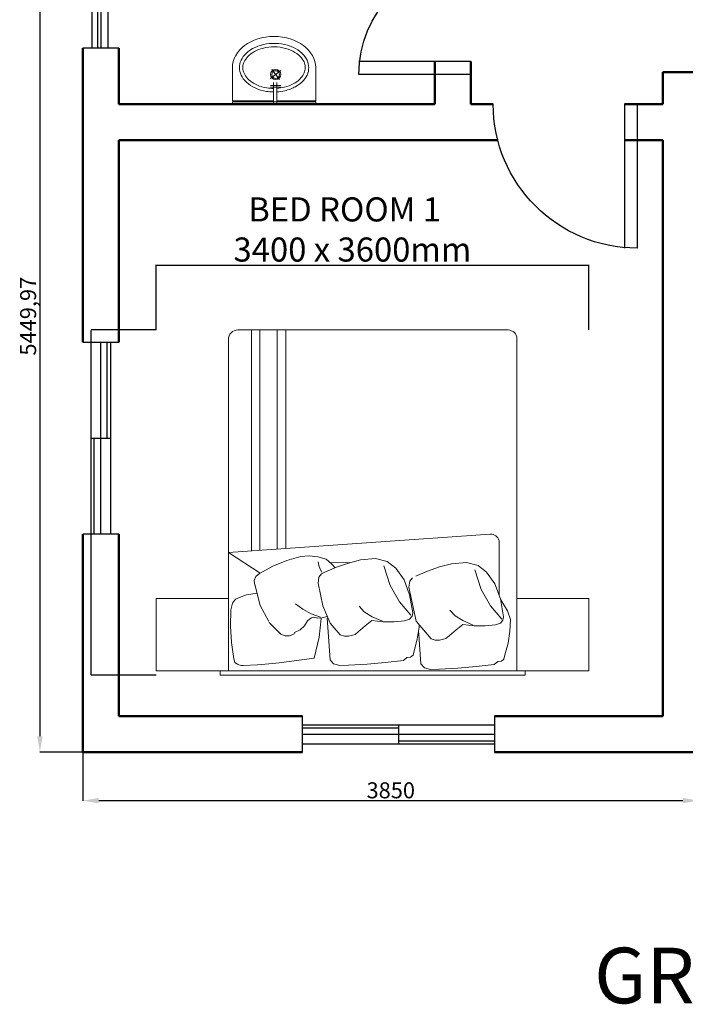
# Model space of a CAD drawing. Units: millimetres. Extents: x -857 to 54106, y -13666 to 13947.
# Tile 2 of 41: x 3174 to 7333, y 2329 to 8482. Entities that reach past the tile are written whole.
import ezdxf

# ---------------------------------------------------------------- set-up
doc = ezdxf.new("R2010")
doc.units = ezdxf.units.MM
for name, color, linetype, lineweight in [('A-ANNO-DIMS', 2, 'Continuous', 18), ('A-ANNO-TEXT', 7, 'Continuous', 25), ('A-AREA-IDEN', 3, 'Continuous', 18), ('A-DOOR', 1, 'Continuous', 25), ('A-FLOR-FIXT', 8, 'Continuous', 18), ('A-FURN', 21, 'Continuous', 18), ('A-FURNITURE', 25, 'Continuous', 9), ('A-GLAZ', 4, 'Continuous', 25), ('A-SANITARY FITTINGS', 25, 'Continuous', 15), ('A-WALL', 7, 'Continuous', 50)]:
    doc.layers.add(name, color=color, linetype=linetype, lineweight=lineweight)
doc.styles.get("Standard").update_dxf_attribs({"font": 'arial.ttf'})
doc.dimstyles.new('ISO-25', dxfattribs={"dimtxt": 2.5, "dimasz": 2.5, "dimexe": 1.25, "dimexo": 0.625, "dimtad": 1, "dimtxsty": 'Standard', "dimcen": 2.5, "dimadec": 0, "dimazin": 0, "dimtfac": 1, "dimtmove": 0, "dimatfit": 3, "dimfxl": 1, "dimarcsym": 0})

# ---------------------------------------------------------------- blocks, each defined once
blk = doc.blocks.new('A$C06e6df2d')
at = {"layer": 'A-FURNITURE'}
for p, q in [((-73.01, 70.89), (-16.87, 70.89)), ((-70.22, 24.92), (-70.22, 70.89)), ((-68.43, 25.04), (-68.43, 70.89)), ((-64.83, 25.3), (-64.83, 70.89)), ((-63.04, 25.42), (-63.04, 70.89)), ((-75.01, 24.58), (-75.01, 68.89)), ((-15.01, 0), (-15.01, 69.09)), ((-75.01, 24.58), (-20.56, 28.42)), ((-18.69, 15.78), (-18.71, 27.06)), ((-68.39, 20.29), (-75.01, 24.58)), ((-75.01, 24.58), (-75.01, 0)), ((-65.73, 21.73), (-62.87, 22.91)), ((-62.87, 22.91), (-59.95, 23.77)), ((-59.95, 23.77), (-58.19, 23.92)), ((-58.19, 23.92), (-56.43, 23.73)), ((-56.43, 23.73), (-54.68, 23.22)), ((-56.16, 21.87), (-56.3, 22.64)), ((-54.68, 23.22), (-54.09, 22.72)), ((-54.09, 22.72), (-53.51, 22.17)), ((-50.02, 22.42), (-47.49, 23.05)), ((-47.49, 23.05), (-44.37, 23.33)), ((-44.37, 23.33), (-41.97, 22.72)), ((-41.97, 22.72), (-40.19, 21.34)), ((-68.53, 20.21), (-65.73, 21.73)), ((-55.9, 21.17), (-56.16, 21.87)), ((-55.54, 20.51), (-55.9, 21.17)), ((-55.62, 20.16), (-54.92, 20.5)), ((-54.92, 20.5), (-52.5, 21.58)), ((-49.77, 22.5), (-53.75, 22.43)), ((-53.51, 22.17), (-52.8, 21.44)), ((-52.5, 21.58), (-50.02, 22.42)), ((-41.32, 17.73), (-42.66, 21.83)), ((-40.19, 21.34), (-38.45, 18.93)), ((-36.02, 19.68), (-33.6, 20.75)), ((-33.6, 20.75), (-31.12, 21.59)), ((-31.12, 21.59), (-28.59, 22.22)), ((-28.59, 22.22), (-25.48, 22.5)), ((-25.48, 22.5), (-23.07, 21.9)), ((-22.42, 16.9), (-23.76, 21)), ((-23.07, 21.9), (-21.29, 20.51)), ((-21.29, 20.51), (-19.55, 18.1)), ((-69.62, 18.81), (-69.3, 19.62)), ((-69.5, 17.78), (-69.62, 18.81)), ((-69.3, 19.62), (-68.53, 20.21)), ((-56.34, 18.24), (-56.19, 19.49)), ((-56.19, 19.49), (-55.62, 20.16)), ((-38.45, 18.93), (-37.3, 15.81)), ((-37.44, 17.41), (-37.29, 18.66)), ((-37.29, 18.66), (-36.72, 19.34)), ((-68.39, 13.59), (-69.52, 17.98)), ((-55.37, 13.49), (-56.34, 18.24)), ((-39.4, 14.32), (-41.32, 17.73)), ((-35.98, 10.29), (-37.44, 17.41)), ((-20.5, 13.49), (-22.42, 16.9)), ((-19.55, 18.1), (-18.4, 14.98)), ((-73.5, 14.91), (-74.12, 14.04)), ((-71.64, 15.67), (-73.5, 14.91)), ((-71.25, 15.78), (-71.44, 15.74)), ((-69.05, 16.16), (-71.23, 15.78)), ((-37.3, 15.81), (-36.66, 12.07)), ((-18.4, 14.98), (-17.76, 11.24)), ((-16.95, 12.45), (-18.35, 14.73)), ((-74.47, 12.68), (-74.56, 9.28)), ((-74.12, 14.04), (-74.47, 12.68)), ((-66.57, 10.23), (-68.39, 13.59)), ((-61.02, 13.94), (-59.51, 12.79)), ((-59.51, 12.79), (-57.79, 11.86)), ((-53.83, 9.92), (-55.37, 13.49)), ((-47.81, 13.43), (-46.76, 12.26)), ((-37.06, 11.55), (-39.4, 14.32)), ((-28.91, 12.6), (-27.86, 11.44)), ((-18.16, 10.72), (-20.5, 13.49)), ((-16.34, 10.65), (-16.95, 12.45)), ((-58.52, 10.37), (-59.16, 9.35)), ((-58.11, 10.75), (-58.52, 10.37)), ((-57.7, 11.01), (-58.11, 10.75)), ((-57.79, 11.86), (-55.84, 11.15)), ((-57.28, 11.14), (-57.7, 11.01)), ((-56.4, 10.96), (-57.28, 11.14)), ((-55.52, 11), (-56.4, 10.96)), ((-56.14, 6.96), (-55.7, 10.85)), ((-54.44, 11.32), (-55.52, 11)), ((-54.44, 10.96), (-53.85, 2.28)), ((-46.76, 12.26), (-45.12, 11.25)), ((-45.15, 10.44), (-46.52, 9.32)), ((-42.78, 10.21), (-45.15, 10.44)), ((-45.12, 11.25), (-42.96, 10.31)), ((-38.37, 10.42), (-40.52, 10.2)), ((-37.33, 10.73), (-38.37, 10.42)), ((-36.79, 11.34), (-37.33, 10.73)), ((-36.66, 12.07), (-36.79, 11.34)), ((-32.85, 6.68), (-35.98, 10.29)), ((-27.86, 11.44), (-26.22, 10.43)), ((-26.22, 10.43), (-24.06, 9.48)), ((-17.89, 10.51), (-18.43, 9.9)), ((-17.76, 11.24), (-17.89, 10.51)), ((-16.43, 8.21), (-16.34, 10.65)), ((-74.56, 9.28), (-74.36, 5.88)), ((-64.09, 7.63), (-66.55, 10.02)), ((-60.04, 8.55), (-61.24, 7.96)), ((-59.16, 9.35), (-60.04, 8.55)), ((-51.75, 7.51), (-53.83, 9.92)), ((-46.52, 9.32), (-47.98, 8.12)), ((-40.52, 10.2), (-42.78, 10.21)), ((-35.72, 6.6), (-35.33, 9.04)), ((-35.43, 8.42), (-34.95, 1.45)), ((-35.33, 9.04), (-35.31, 9.52)), ((-27.62, 8.5), (-29.08, 7.29)), ((-26.26, 9.61), (-27.62, 8.5)), ((-23.88, 9.38), (-26.26, 9.61)), ((-21.62, 9.38), (-23.88, 9.38)), ((-19.47, 9.59), (-21.62, 9.38)), ((-18.43, 9.9), (-19.47, 9.59)), ((-16.82, 5.77), (-16.43, 8.21)), ((-63.18, 7.26), (-64.09, 7.63)), ((-62.27, 7.28), (-63.18, 7.26)), ((-61.35, 7.68), (-62.27, 7.28)), ((-61.24, 7.96), (-61.35, 7.68)), ((-57.17, 2.61), (-56.14, 6.96)), ((-50.88, 7.2), (-51.75, 7.51)), ((-50.02, 7.17), (-50.88, 7.2)), ((-49.15, 7.42), (-50.02, 7.17)), ((-48.66, 7.55), (-49.15, 7.42)), ((-47.98, 8.12), (-48.66, 7.55)), ((-36.37, 4.16), (-35.72, 6.6)), ((-31.98, 6.37), (-32.85, 6.68)), ((-31.12, 6.34), (-31.98, 6.37)), ((-30.25, 6.59), (-31.12, 6.34)), ((-29.76, 6.73), (-30.25, 6.59)), ((-29.08, 7.29), (-29.76, 6.73)), ((-74.36, 5.88), (-73.9, 2.49)), ((-36.6, 3.27), (-36.37, 4.16)), ((-17.47, 3.33), (-16.82, 5.77)), ((-73.9, 2.49), (-73.65, 1.74)), ((-64.46, 1.68), (-60.83, 2.11)), ((-60.83, 2.11), (-57.17, 2.61)), ((-53.85, 2.28), (-53.12, 1.45)), ((-42.37, 1.69), (-38.61, 2.15)), ((-38.61, 2.15), (-37.87, 2.73)), ((-37.87, 2.73), (-37.09, 2.83)), ((-37.09, 2.83), (-36.6, 3.27)), ((-18.19, 2.01), (-17.71, 2.44)), ((-17.71, 2.44), (-17.47, 3.33)), ((-76.74, 0), (-76.74, -0.9)), ((-13.27, 0), (-76.74, 0)), ((-73.65, 1.74), (-73.12, 1.41)), ((-71.96, 1.11), (-68.94, 1.26)), ((-68.94, 1.26), (-68.06, 1.33)), ((-68.06, 1.33), (-64.46, 1.68)), ((-53.12, 1.45), (-51.84, 1.07)), ((-51.84, 1.07), (-49.99, 1.14)), ((-49.99, 1.14), (-46.17, 1.35)), ((-46.17, 1.35), (-42.37, 1.69)), ((-34.95, 1.45), (-34.22, 0.63)), ((-34.22, 0.63), (-32.94, 0.25)), ((-32.94, 0.25), (-31.09, 0.31)), ((-31.09, 0.31), (-27.27, 0.52)), ((-27.27, 0.52), (-23.47, 0.86)), ((-23.47, 0.86), (-19.71, 1.32)), ((-19.71, 1.32), (-18.97, 1.91)), ((-18.97, 1.91), (-18.19, 2.01)), ((-13.27, -0.9), (-13.27, 0)), ((-13.27, -0.9), (-76.74, -0.9))]:
    blk.add_line(p, q, dxfattribs=at)
for points in [[(-75.01, 0), (-90.01, 0), (-90.01, 15.01), (-75.01, 15.01)], [(-15.01, 0), (0, 0), (0, 15.01), (-15.01, 15.01)]]:
    blk.add_lwpolyline(points, close=True, dxfattribs=at)
for centre, radius, start, end in [((-73.01, 68.89), 2, 90, 180), ((-16.8, 69.09), 1.8, 0, 90), ((-20.45, 26.63), 1.8, 13.7792, 93.47), ((-70.89, 13.81), 2, 99.8546, 112.1195), ((-72.06, 3.1), 2, 238.0354, 272.9353)]:
    blk.add_arc(centre, radius, start, end, dxfattribs=at)
blk = doc.blocks.new('A$C0124305E')
at = {"layer": 'A-SANITARY FITTINGS'}
for p, q in [((-8.42, 16.01), (-0.8, 16.01)), ((-0.8, 7.08), (-0.8, 16.01)), ((-5.66, 7.68), (-8, 5.88)), ((-7.73, 7.95), (-5.93, 5.62)), ((0, 7.08), (-4.99, 7.08)), ((-4.31, 5.61), (-4.31, 7.96)), ((-3.91, 5.61), (-3.91, 7.96)), ((0, 6.28), (-4.99, 6.28)), ((-0.8, -3.19), (-0.8, 6.28)), ((-8.42, -3.19), (-0.8, -3.19))]:
    blk.add_line(p, q, dxfattribs=at)
blk.add_lwpolyline([(-0.5, 16.01), (0, 16.01), (0, -3.19), (-0.5, -3.19)], close=True, dxfattribs=at)
for radius in [1.18, 0.885]:
    blk.add_circle((-6.83, 6.78), radius, dxfattribs=at)
at = {"layer": 'A-SANITARY FITTINGS', "extrusion": (0, 0, -1)}
blk.add_ellipse((-8.42, 6.41), major_axis=(0, 9.6), ratio=0.75, start_param=3.141593, end_param=6.283185, dxfattribs=at)
at = {"layer": 'A-SANITARY FITTINGS'}
for points, knots in [([(-2.82, 6.28), (-2.82, 5.74), (-2.87, 5.2), (-3.1, 3.74), (-3.37, 2.86), (-4.09, 1.28), (-4.55, 0.6), (-5.56, -0.5), (-6.12, -0.92), (-7.25, -1.45), (-7.83, -1.58), (-8.98, -1.59), (-9.55, -1.46), (-10.69, -0.93), (-11.25, -0.52), (-12.27, 0.57), (-12.72, 1.25), (-13.45, 2.82), (-13.72, 3.71), (-14.02, 5.56), (-14.05, 6.52), (-13.88, 8.41), (-13.67, 9.32), (-13.04, 10.99), (-12.62, 11.73), (-11.66, 12.96), (-11.12, 13.45), (-10, 14.13), (-9.43, 14.32), (-8.28, 14.45), (-7.7, 14.39), (-6.56, 14), (-5.99, 13.66), (-4.93, 12.71), (-4.44, 12.09), (-3.62, 10.62), (-3.3, 9.78), (-2.96, 8.29), (-2.87, 7.69), (-2.84, 7.08)], [1.58652, 1.58652, 1.58652, 1.58652, 1.780321, 1.780321, 2.120053, 2.120053, 2.459785, 2.459785, 2.799517, 2.799517, 3.139249, 3.139249, 3.478981, 3.478981, 3.818713, 3.818713, 4.158445, 4.158445, 4.498177, 4.498177, 4.837909, 4.837909, 5.177641, 5.177641, 5.517373, 5.517373, 5.857105, 5.857105, 6.196837, 6.196837, 6.536569, 6.536569, 6.876301, 6.876301, 7.216033, 7.216033, 7.555765, 7.555765, 7.774364, 7.774364, 7.774364, 7.774364]), ([(-3.62, 6.29), (-3.62, 5.76), (-3.67, 5.23), (-3.88, 3.96), (-4.1, 3.23), (-4.65, 1.95), (-4.98, 1.39), (-5.72, 0.46), (-6.12, 0.1), (-6.92, -0.44), (-7.32, -0.61), (-8.11, -0.8), (-8.5, -0.81), (-9.28, -0.69), (-9.68, -0.55), (-10.48, -0.08), (-10.89, 0.24), (-11.67, 1.13), (-12.05, 1.7), (-12.66, 3.01), (-12.9, 3.76), (-13.2, 5.38), (-13.25, 6.28), (-13.13, 8.02), (-12.95, 8.88), (-12.42, 10.42), (-12.06, 11.12), (-11.23, 12.25), (-10.77, 12.7), (-9.92, 13.26), (-9.53, 13.43), (-8.78, 13.62), (-8.41, 13.64), (-7.66, 13.54), (-7.28, 13.42), (-6.51, 13.02), (-6.12, 12.73), (-5.35, 11.95), (-4.97, 11.43), (-4.34, 10.23), (-4.08, 9.54), (-3.76, 8.24), (-3.67, 7.64), (-3.63, 7.03)], [1.58652, 1.58652, 1.58652, 1.58652, 1.790653, 1.790653, 2.093007, 2.093007, 2.384527, 2.384527, 2.676047, 2.676047, 2.967567, 2.967567, 3.259087, 3.259087, 3.550608, 3.550608, 3.842128, 3.842128, 4.155456, 4.155456, 4.468784, 4.468784, 4.806699, 4.806699, 5.144614, 5.144614, 5.482529, 5.482529, 5.820444, 5.820444, 6.099515, 6.099515, 6.378586, 6.378586, 6.657656, 6.657656, 6.936727, 6.936727, 7.23864, 7.23864, 7.540552, 7.540552, 7.774364, 7.774364, 7.774364, 7.774364])]:
    blk.add_open_spline(points, degree=3, knots=knots, dxfattribs=at)
blk = doc.blocks.new('*D23')
at = {"layer": 'A-ANNO-DIMS', "color": 0, "lineweight": -2, "transparency": 16777216}
for p, q in [((3566.7, 9354.2), (3298.9, 9354.2)), ((3300.1, 9254.2), (3300.1, 4004.3)), ((3566, 3904.3), (3298.9, 3904.3))]:
    blk.add_line(p, q, dxfattribs=at)
at = {"layer": 'A-ANNO-DIMS', "color": 0, "transparency": 16777216}
for points in [[(3283.5, 9254.2), (3316.8, 9254.2), (3300.1, 9354.2)], [(3283.5, 4004.3), (3316.8, 4004.3), (3300.1, 3904.3)]]:
    blk.add_solid(points, dxfattribs=at)
at = {"layer": 'Defpoints', "color": 0, "transparency": 16777216}
for p in [(3567.3, 9354.2), (3300.1, 3904.3), (3566.6, 3904.3)]:
    blk.add_point(p, dxfattribs=at)
at = {"layer": 'A-ANNO-DIMS', "color": 0, "transparency": 16777216, "insert": (3239.4, 6629.2), "char_height": 100, "attachment_point": 5, "rotation": 90}
blk.add_mtext('5449,97', dxfattribs=at)
blk = doc.blocks.new('*D24')
at = {"layer": 'A-ANNO-DIMS', "color": 0, "lineweight": -2, "transparency": 16777216}
for p, q in [((3567.3, 3903.6), (3567.3, 3600.6)), ((7417.3, 3903.2), (7417.3, 3600.6)), ((3667.3, 3601.8), (7317.3, 3601.8))]:
    blk.add_line(p, q, dxfattribs=at)
at = {"layer": 'A-ANNO-DIMS', "color": 0, "transparency": 16777216}
for points in [[(3667.3, 3618.5), (3667.3, 3585.1), (3567.3, 3601.8)], [(7317.3, 3618.5), (7317.3, 3585.1), (7417.3, 3601.8)]]:
    blk.add_solid(points, dxfattribs=at)
at = {"layer": 'Defpoints', "color": 0, "transparency": 16777216}
for p in [(3567.3, 3904.3), (7417.3, 3903.8), (7417.3, 3601.8)]:
    blk.add_point(p, dxfattribs=at)
at = {"layer": 'A-ANNO-DIMS', "color": 0, "transparency": 16777216, "insert": (5492.3, 3653.5), "char_height": 100, "attachment_point": 5}
blk.add_mtext('3850', dxfattribs=at)
blk = doc.blocks.new('DOOR-900')
blk.add_line((11417.3, 9811.5), (12317.3, 9811.5))
blk.add_arc((11417.3, 9811.5), 900, 0, 90)
blk = doc.blocks.new('DOOR-700')
blk.add_line((8245.5, 10779.2), (8245.5, 11479.2))
blk.add_arc((8245.5, 10779.2), 700, 90, 180)
blk = doc.blocks.new('WIN-1200')
for p, q in [((9371.3, 11750.2), (10571.3, 11750.2)), ((9371.3, 11731.7), (9971.3, 11731.7)), ((9371.3, 11691.7), (10571.3, 11691.7)), ((9971.3, 11750.2), (9971.3, 11630.7)), ((10571.3, 11630.7), (9371.3, 11630.7)), ((9971.3, 11651.7), (10571.3, 11651.7))]:
    blk.add_line(p, q)
for points in [[(9371.3, 11579.2), (9371.3, 11804.2)], [(10571.3, 11804.2), (10571.3, 11579.2)]]:
    blk.add_lwpolyline(points)
blk = doc.blocks.new('WIN-700')
for p, q in [((3626.3, 8304.2), (3626.3, 9004.2)), ((3679.8, 9004.2), (3679.8, 8304.2)), ((3699.8, 9004.2), (3699.8, 8654.2)), ((3724.4, 9004.2), (3724.4, 8304.2)), ((3724.4, 8654.2), (3626.3, 8654.2)), ((3659.8, 8654.2), (3659.8, 8304.2))]:
    blk.add_line(p, q)
for points in [[(3567.3, 9004.2), (3792.3, 9004.2)], [(3792.3, 8304.2), (3567.3, 8304.2)]]:
    blk.add_lwpolyline(points)
blk = doc.blocks.new('*D45')
at = {"layer": 'A-ANNO-DIMS', "color": 0, "lineweight": -2, "transparency": 16777216}
for p, q in [((4026.8, 6543.6), (4026.8, 6949.8)), ((4029.3, 6948.6), (6728.4, 6948.6)), ((6730.9, 6543.6), (6730.9, 6949.8))]:
    blk.add_line(p, q, dxfattribs=at)
at = {"layer": 'A-ANNO-DIMS', "color": 0, "transparency": 16777216}
for points in [[(4029.3, 6949), (4029.3, 6948.2), (4026.8, 6948.6)], [(6728.4, 6949), (6728.4, 6948.2), (6730.9, 6948.6)]]:
    blk.add_solid(points, dxfattribs=at)
at = {"layer": 'Defpoints', "color": 0, "transparency": 16777216}
for p in [(6730.9, 6948.6), (4026.8, 6543), (6730.9, 6543)]:
    blk.add_point(p, dxfattribs=at)
at = {"layer": 'A-ANNO-DIMS', "color": 0, "transparency": 16777216, "insert": (5378.8, 6950.5), "char_height": 2.5, "attachment_point": 5}
blk.add_mtext('DOUBLE BED 2704', dxfattribs=at)
blk = doc.blocks.new('*D46')
at = {"layer": 'A-ANNO-DIMS', "color": 0, "lineweight": -2, "transparency": 16777216}
for p, q in [((4026.2, 6543), (3619.9, 6543)), ((3621.2, 4388.9), (3621.2, 6540.5)), ((4026.2, 4386.4), (3619.9, 4386.4))]:
    blk.add_line(p, q, dxfattribs=at)
at = {"layer": 'A-ANNO-DIMS', "color": 0, "transparency": 16777216}
for points in [[(3620.8, 6540.5), (3621.6, 6540.5), (3621.2, 6543)], [(3620.8, 4388.9), (3621.6, 4388.9), (3621.2, 4386.4)]]:
    blk.add_solid(points, dxfattribs=at)
at = {"layer": 'Defpoints', "color": 0, "transparency": 16777216}
for p in [(3621.2, 6543), (4026.8, 6543), (4026.8, 4386.4)]:
    blk.add_point(p, dxfattribs=at)
at = {"layer": 'A-ANNO-DIMS', "color": 0, "transparency": 16777216, "insert": (3619.3, 5464.7), "char_height": 2.5, "attachment_point": 5, "rotation": 90}
blk.add_mtext('2157', dxfattribs=at)

msp = doc.modelspace()

# ---------------------------------------------------------------- linework, layer by layer
at = {"layer": 'A-DOOR'}
for p, q in [((5992.28, 8220.088), (5292.28, 8220.088)), ((5992.28, 8140.088), (5992.28, 8220.088)), ((5992.28, 8140.088), (5992.28, 8220.088)), ((6952.158, 7954.231), (6952.158, 7054.231))]:
    msp.add_line(p, q, dxfattribs=at)
at = {"layer": 'A-WALL'}
for p, q in [((3792.28, 8304.231), (3792.28, 7954.231)), ((5767.28, 7954.231), (5767.28, 8220.088)), ((5992.28, 7954.231), (5992.28, 8220.088)), ((7192.28, 8154.231), (7417.28, 8154.231)), ((7192.28, 8154.231), (7192.28, 7954.231)), ((3792.28, 7954.231), (5767.28, 7954.231)), ((6132.158, 7954.231), (5992.28, 7954.231)), ((7192.28, 7954.231), (6952.158, 7954.231)), ((3792.28, 7729.231), (6160.737, 7729.231)), ((3792.28, 6467.586), (3792.28, 7729.231)), ((6952.158, 7729.231), (7192.28, 7729.231)), ((7192.28, 7729.231), (7192.28, 4129.231)), ((3792.28, 4129.231), (3792.28, 5267.586)), ((3792.28, 4129.231), (4940.719, 4129.231)), ((6140.719, 4129.023), (7192.28, 4129.231)), ((6140.719, 3904.023), (7417.28, 3904.023))]:
    msp.add_line(p, q, dxfattribs=at)
for points in [[(3567.28, 6467.586), (3567.28, 8304.231)], [(4940.719, 3904.094), (3567.28, 3904.258), (3567.28, 5267.586)]]:
    msp.add_lwpolyline(points, dxfattribs=at)

# ---------------------------------------------------------------- block references
at = {"layer": 'A-DOOR', "extrusion": (0, 0, -1), "zscale": -1, "rotation": 269.9999999999999}
for name, p in [('DOOR-700', (-16771.511, 16385.634)), ('DOOR-900', (-16843.639, 19371.511))]:
    msp.add_blockref(name, p, dxfattribs=at)
at = {"layer": 'A-FLOR-FIXT', "xscale": 27.10344997005861, "yscale": 27.10344997005861, "zscale": 27.10344997005861, "rotation": 270.0000000004072}
msp.add_blockref('A$C0124305E', (4589.284, 7954.231), dxfattribs=at)
at = {"layer": 'A-FURN', "xscale": 30.0410247625267, "yscale": 30.0410247625267, "zscale": 30.0410247625267}
msp.add_blockref('A$C06e6df2d', (6730.869, 4413.34), dxfattribs=at)
at = {"layer": 'A-GLAZ'}
for name, p in [('WIN-700', (0, 0)), ('WIN-1200', (-4430.622, -7675.208))]:
    msp.add_blockref(name, p, dxfattribs=at)
at = {"layer": 'A-GLAZ', "rotation": 89.99999999999982}
msp.add_blockref('WIN-1200', (15371.511, -4103.754), dxfattribs=at)

# ---------------------------------------------------------------- texts
at = {"layer": 'A-ANNO-TEXT', "insert": (6763.058, 2682.963), "char_height": 347.60543, "attachment_point": 1}
msp.add_mtext_dynamic_manual_height_columns('\\pxt0;GROUND FLOOR PLAN', width=5900.0263, gutter_width=43450.679, heights=[5996.136], dxfattribs=at)
at = {"layer": 'A-AREA-IDEN', "insert": (4509.517, 7371.736), "char_height": 150.48461, "attachment_point": 1}
msp.add_mtext_dynamic_manual_height_columns('\\pxt0;  BED ROOM 1\\P3400 x 3600mm', width=2554.22693, gutter_width=18810.576, heights=[2595.835], dxfattribs=at)

# ---------------------------------------------------------------- dimensions: what is measured, and where the dimension line sits
at = {"layer": 'A-ANNO-DIMS'}
for base, p1, p2, override, picture, middle in [((3300.128, 3904.258), (3567.28, 9354.231), (3566.631, 3904.258), {"dimtxt": 100, "dimasz": 100, "dimclrd": 0, "dimclre": 0, "dimclrt": 0}, '*D23', (3239.407, 6629.244)), ((3621.187, 6542.981), (4026.797, 4386.352), (4026.797, 6542.981), {"dimdec": 0, "dimrnd": 0, "dimzin": 0, "dimlunit": 2}, '*D46', (3619.285, 5464.666))]:
    dim = msp.add_linear_dim(base=base, p1=p1, p2=p2, angle=90, dimstyle='ISO-25', override=override, dxfattribs=at)
    dim.commit()
    dim.dimension.update_dxf_attribs({"geometry": picture, "text_midpoint": middle})
dim = msp.add_linear_dim(base=(6730.869, 6948.592), p1=(4026.797, 6542.981), p2=(6730.869, 6542.981), text='DOUBLE BED <>', dimstyle='ISO-25', override={"dimdec": 0, "dimrnd": 0, "dimzin": 0, "dimlunit": 2}, dxfattribs=at)
dim.commit()
dim.dimension.update_dxf_attribs({"geometry": '*D45', "text_midpoint": (5378.833, 6950.51)})
dim = msp.add_linear_dim(base=(7417.28, 3601.816), p1=(3567.28, 3904.258), p2=(7417.28, 3903.799), dimstyle='ISO-25', override={"dimtxt": 100, "dimasz": 100, "dimclrd": 0, "dimclre": 0, "dimclrt": 0}, dxfattribs=at)
dim.commit()
dim.dimension.update_dxf_attribs({"geometry": '*D24', "text_midpoint": (5492.28, 3653.533)})

doc.saveas('drawing.dxf')
